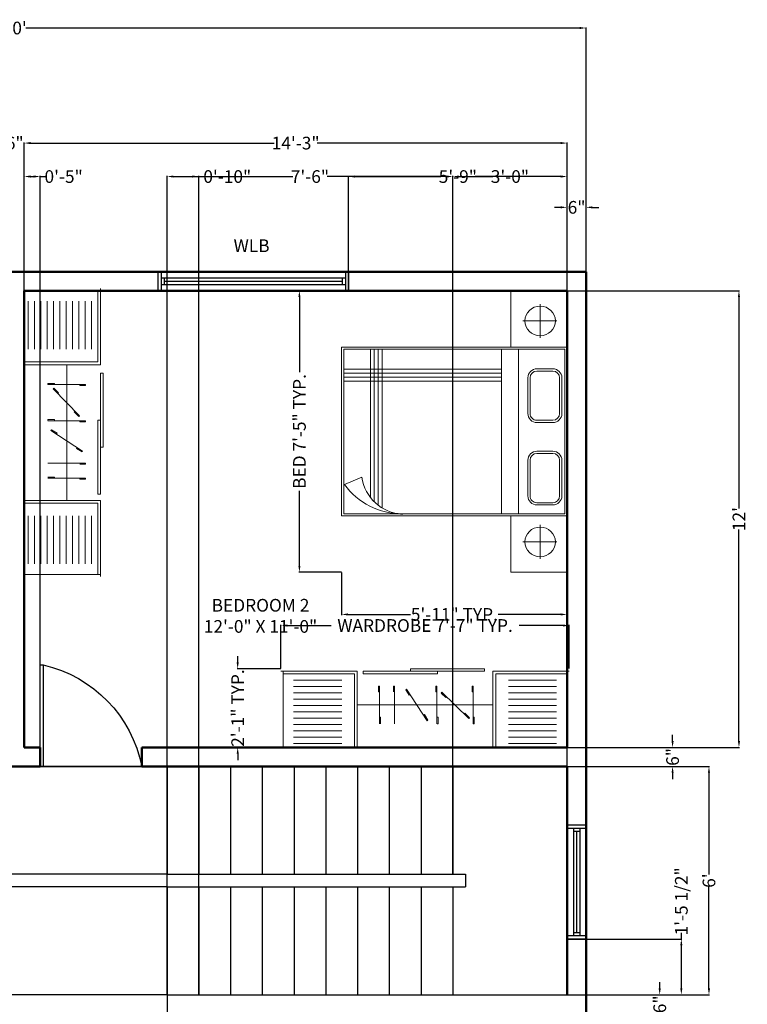
# Model space of a CAD drawing. Units: inches. Extents: x 2663 to 3147, y 140 to 736.
# Tile 6 of 6: x 2918 to 3147, y 425 to 736. Entities that reach past the tile are written whole.
import ezdxf

# ---------------------------------------------------------------- set-up
doc = ezdxf.new("R2010")
doc.units = ezdxf.units.IN
doc.header["$MEASUREMENT"] = 0
for name, color, linetype, lineweight in [('A-ANNO-DIMS', 2, 'Continuous', 18), ('A-AREA-IDEN', 3, 'Continuous', 25), ('A-DOOR', 3, 'Continuous', 25), ('A-FLOR-STRS', 1, 'Continuous', 25), ('A-FURN', 8, 'Continuous', 18), ('A-GLAZ', 4, 'Continuous', 25), ('A-WALL', 7, 'Continuous', 50)]:
    doc.layers.add(name, color=color, linetype=linetype, lineweight=lineweight)
doc.styles.get("Standard").update_dxf_attribs({"font": 'arial.ttf'})
doc.dimstyles.get("Standard").update_dxf_attribs({"dimtxt": 4, "dimasz": 2, "dimexe": 0.18, "dimexo": 0.0625, "dimgap": 0.09, "dimtad": 0, "dimdec": 0, "dimzin": 0, "dimdsep": 46, "dimlunit": 4, "dimtxsty": 'Standard', "dimcen": 0.09, "dimadec": 0, "dimazin": 0, "dimtfac": 1, "dimtdec": 0, "dimtofl": 0, "dimtmove": 0, "dimatfit": 3, "dimfxl": 1, "dimtolj": 1, "dimtzin": 0, "dimarcsym": 0})

# ---------------------------------------------------------------- blocks, each defined once
blk = doc.blocks.new('*D2')
at = {"layer": 'A-ANNO-DIMS', "color": 0, "lineweight": -2, "transparency": 16777216}
for p, q in [((2911.16, 696.87), (2909.16, 696.87)), ((2913.16, 650.39), (2913.16, 697.05)), ((2919.16, 650.39), (2919.16, 697.05)), ((2921.16, 696.87), (2923.16, 696.87))]:
    blk.add_line(p, q, dxfattribs=at)
at = {"layer": 'A-ANNO-DIMS', "color": 0, "transparency": 16777216}
for points in [[(2911.16, 697.21), (2911.16, 696.54), (2913.16, 696.87)], [(2921.16, 697.21), (2921.16, 696.54), (2919.16, 696.87)]]:
    blk.add_solid(points, dxfattribs=at)
at = {"layer": 'Defpoints', "color": 0, "transparency": 16777216}
for p in [(2919.16, 696.87), (2913.16, 650.32), (2919.16, 650.32)]:
    blk.add_point(p, dxfattribs=at)
at = {"layer": 'A-ANNO-DIMS', "color": 0, "transparency": 16777216, "insert": (2916.16, 696.87), "char_height": 4, "attachment_point": 5}
blk.add_mtext('\\A1;6"', dxfattribs=at)
blk = doc.blocks.new('*D3')
at = {"layer": 'A-ANNO-DIMS', "color": 0, "lineweight": -2, "transparency": 16777216}
for p, q in [((2919.16, 650.39), (2919.16, 697.05)), ((2921.16, 696.87), (2997.89, 696.87)), ((3088.16, 696.87), (3011.43, 696.87)), ((3090.16, 650.39), (3090.16, 697.05))]:
    blk.add_line(p, q, dxfattribs=at)
at = {"layer": 'A-ANNO-DIMS', "color": 0, "transparency": 16777216}
for points in [[(2921.16, 697.21), (2921.16, 696.54), (2919.16, 696.87)], [(3088.16, 697.21), (3088.16, 696.54), (3090.16, 696.87)]]:
    blk.add_solid(points, dxfattribs=at)
at = {"layer": 'Defpoints', "color": 0, "transparency": 16777216}
for p in [(3090.16, 696.87), (2919.16, 650.32), (3090.16, 650.32)]:
    blk.add_point(p, dxfattribs=at)
at = {"layer": 'A-ANNO-DIMS', "color": 0, "transparency": 16777216, "insert": (3004.66, 696.87), "char_height": 4, "attachment_point": 5}
blk.add_mtext('\\A1;14\'-3"', dxfattribs=at)
blk = doc.blocks.new('*D7')
at = {"layer": 'A-ANNO-DIMS', "color": 0, "lineweight": -2, "transparency": 16777216}
for p, q in [((3090.22, 500.32), (3135.04, 500.32)), ((3134.86, 498.32), (3134.86, 466.26)), ((3134.86, 430.32), (3134.86, 462.38)), ((3090.22, 428.32), (3135.04, 428.32))]:
    blk.add_line(p, q, dxfattribs=at)
at = {"layer": 'A-ANNO-DIMS', "color": 0, "transparency": 16777216}
for points in [[(3134.53, 498.32), (3135.2, 498.32), (3134.86, 500.32)], [(3134.53, 430.32), (3135.2, 430.32), (3134.86, 428.32)]]:
    blk.add_solid(points, dxfattribs=at)
at = {"layer": 'Defpoints', "color": 0, "transparency": 16777216}
for p in [(3090.16, 500.32), (3090.16, 428.32), (3134.86, 428.32)]:
    blk.add_point(p, dxfattribs=at)
at = {"layer": 'A-ANNO-DIMS', "color": 0, "transparency": 16777216, "insert": (3134.86, 464.32), "char_height": 4, "attachment_point": 5, "rotation": 90}
blk.add_mtext("\\A1;6'", dxfattribs=at)
blk = doc.blocks.new('EDFRTYUI')
for p, q in [((3325.9, 253.54), (3325.9, 259.54)), ((3325.9, 259.54), (3385.9, 259.54)), ((3326.9, 253.54), (3326.9, 259.54)), ((3384.9, 259.54), (3384.9, 253.54)), ((3385.9, 259.54), (3385.9, 253.54)), ((3326.9, 257.54), (3384.9, 257.54)), ((3326.9, 255.54), (3384.9, 255.54)), ((3327.9, 255.54), (3327.9, 257.54)), ((3327.9, 256.54), (3383.9, 256.54)), ((3383.9, 257.54), (3383.9, 255.54)), ((3385.9, 253.54), (3325.9, 253.54))]:
    blk.add_line(p, q)
at = {"insert": (3337.87, 269.72), "char_height": 4, "attachment_point": 1}
blk.add_mtext_dynamic_manual_height_columns('\\pxqc;WLB', width=34.9199, gutter_width=20, heights=[0], dxfattribs=at)
blk = doc.blocks.new('FGCHBJK')
for p, q in [((3315.88, 342.07), (3315.88, 348.07)), ((3315.88, 348.07), (3351.88, 348.07)), ((3316.88, 342.07), (3316.88, 348.07)), ((3350.88, 348.07), (3350.88, 342.07)), ((3351.88, 348.07), (3351.88, 342.07)), ((3316.88, 346.07), (3350.88, 346.07)), ((3317.88, 344.07), (3317.88, 346.07)), ((3317.88, 345.07), (3349.88, 345.07)), ((3349.88, 346.07), (3349.88, 344.07)), ((3351.88, 342.07), (3315.88, 342.07)), ((3316.88, 344.07), (3350.88, 344.07))]:
    blk.add_line(p, q)
blk = doc.blocks.new('A$C057D194F')
for p, q in [((0, 1.5, -0.1688), (0, 2, -0.1688)), ((0, 2, -0.1688), (0.5, 2, -0.1688)), ((0.5, 2, -0.1688), (0.5, 0, -0.1688)), ((2, 2, -0.1688), (0.5, 2, -0.1688)), ((1.98, 1.98, -0.1688), (0.52, 1.98, -0.1688)), ((0.52, 1.98, -0.1688), (0.52, 0.02, -0.1688)), ((1.0907, 1.9539, -0.1688), (0.7735, 1.9539, -0.1688)), ((1.0907, 1.9339, -0.1688), (0.7735, 1.9339, -0.1688)), ((1.8224, 1.9539, -0.1688), (1.5052, 1.9539, -0.1688)), ((1.8224, 1.9339, -0.1688), (1.5052, 1.9339, -0.1688)), ((1.98, 0.02, -0.1688), (1.98, 1.98, -0.1688)), ((2, 0, -0.1688), (2, 2, -0.1688)), ((2.5, 2, -0.1688), (2, 2, -0.1688)), ((2.5, 1.5, -0.1688), (2.5, 2, -0.1688)), ((0.2687, 1.9081, -0.1688), (0.2687, 1.761, -0.1688)), ((0.2687, 1.6081, -0.1688), (0.2687, 1.9081, -0.1688)), ((0.6935, 1.8739, -0.1688), (0.6935, 1.7322, -0.1688)), ((0.7135, 1.8739, -0.1688), (0.7135, 1.7322, -0.1688)), ((1.1507, 1.7322, -0.1688), (1.1507, 1.8739, -0.1688)), ((1.1707, 1.7322, -0.1688), (1.1707, 1.8739, -0.1688)), ((1.4252, 1.8739, -0.1688), (1.4252, 1.7322, -0.1688)), ((1.4452, 1.8739, -0.1688), (1.4452, 1.7322, -0.1688)), ((1.8824, 1.7322, -0.1688), (1.8824, 1.8739, -0.1688)), ((1.9024, 1.7322, -0.1688), (1.9024, 1.8739, -0.1688)), ((2.2313, 1.9081, -0.1688), (2.2313, 1.761, -0.1688)), ((2.2313, 1.6081, -0.1688), (2.2313, 1.9081, -0.1688)), ((0.4194, 1.761, -0.1688), (0.1194, 1.761, -0.1688)), ((0.2687, 1.761, -0.1688), (0.4194, 1.761, -0.1688)), ((0.2687, 1.761, -0.1688), (0.2687, 1.6081, -0.1688)), ((2.0806, 1.761, -0.1688), (2.3806, 1.761, -0.1688)), ((2.2313, 1.761, -0.1688), (2.0806, 1.761, -0.1688)), ((2.2313, 1.761, -0.1688), (2.2313, 1.6081, -0.1688)), ((0.7735, 1.6722, -0.1688), (1.0907, 1.6722, -0.1688)), ((1.5052, 1.6722, -0.1688), (1.8224, 1.6722, -0.1688)), ((0.7735, 1.6522, -0.1688), (1.0907, 1.6522, -0.1688)), ((1.5052, 1.6522, -0.1688), (1.8224, 1.6522, -0.1688)), ((0.5, 1.5, -0.1688), (0, 1.5, -0.1688)), ((1.98, 1.5693, -0.1688), (0.52, 1.5693, -0.1688)), ((2, 1.5, -0.1688), (2.5, 1.5, -0.1688)), ((1.98, 1.4193, -0.1688), (0.52, 1.4193, -0.1688)), ((0.6969, 0.02, -0.1688), (0.6969, 1.4193, -0.1688)), ((0.7319, 0.02, -0.1688), (0.7319, 1.4193, -0.1688)), ((0.7669, 0.02, -0.1688), (0.7669, 1.4193, -0.1688)), ((0.8019, 0.02, -0.1688), (0.8019, 1.4193, -0.1688)), ((0.52, 0.3595, -0.1688), (1.9292, 0.3595, -0.1688)), ((0.52, 0.3245, -0.1688), (1.905, 0.3245, -0.1688)), ((0.52, 0.2895, -0.1688), (1.8742, 0.2895, -0.1688)), ((0.52, 0.2545, -0.1688), (1.8344, 0.2545, -0.1688)), ((1.6548, 0.1789, -0.1688), (1.7198, 0.0251, -0.1688)), ((0.52, 0.02, -0.1688), (1.98, 0.02, -0.1688)), ((0.5, 0, -0.1688), (2, 0, -0.1688))]:
    blk.add_line(p, q)
for centre, radius, start, end in [((0.7735, 1.8739, -0.1688), 0.08, 90, 180), ((0.7735, 1.8739, -0.1688), 0.06, 90, 180), ((1.0907, 1.8739, -0.1688), 0.08, 0, 90), ((1.0907, 1.8739, -0.1688), 0.06, 0, 90), ((1.5052, 1.8739, -0.1688), 0.08, 90, 180), ((1.5052, 1.8739, -0.1688), 0.06, 90, 180), ((1.8224, 1.8739, -0.1688), 0.08, 0, 90), ((1.8224, 1.8739, -0.1688), 0.06, 0, 90), ((0.7735, 1.7322, -0.1688), 0.08, 180, 270), ((0.7735, 1.7322, -0.1688), 0.06, 180, 270), ((1.0907, 1.7322, -0.1688), 0.08, 270, 0), ((1.0907, 1.7322, -0.1688), 0.06, 270, 0), ((1.5052, 1.7322, -0.1688), 0.08, 180, 270), ((1.5052, 1.7322, -0.1688), 0.06, 180, 270), ((1.8224, 1.7322, -0.1688), 0.08, 270, 0), ((1.8224, 1.7322, -0.1688), 0.06, 270, 0), ((1.5992, 0.5623, -0.1688), 0.3874, 278.2518, 356.6808), ((1.363, 0.5286, -0.1688), 0.6171, 305.32946, 1.04595)]:
    blk.add_arc(centre, radius, start, end)
blk.add_ellipse((0.2687, 1.761, -0.1688), major_axis=(0, -0.1351), ratio=0.975448)
at = {"extrusion": (0, 0, -1)}
blk.add_ellipse((2.2313, 1.761, -0.1688), major_axis=(0, 0.1351), ratio=0.975448, dxfattribs=at)
for p in [(0.2687, 1.761, -0.1688), (2.2313, 1.761, -0.1688)]:
    blk.add_point(p)
blk = doc.blocks.new('A$C34930FF8')
at = {"ltscale": 0.05}
for p, q in [((0, 2252.4), (0, 16.8)), ((600, 2252.4), (0, 2252.4)), ((185.4, 1513), (185.4, 1521.5)), ((227.1, 1479.2), (233.2, 1485.2)), ((237.7, 1513), (237.7, 1521.5)), ((436.7, 1513), (436.7, 1504.4)), ((482.5, 1513), (482.5, 1504.4)), ((263.6, 1441.7), (269.7, 1447.7)), ((398.2, 1303.6), (392.1, 1297.6)), ((434.8, 1266.1), (428.7, 1260.1)), ((185.4, 1229.1), (185.4, 1237.7)), ((237.7, 1229.1), (237.7, 1237.7)), ((436.7, 1228.2), (436.7, 1219.7)), ((482.5, 1228.2), (482.5, 1219.7)), ((209.5, 1150.1), (214.1, 1157.3)), ((253.5, 1121.8), (258.1, 1129)), ((415.3, 1017.6), (410.6, 1010.5)), ((459.3, 989.3), (454.7, 982.1)), ((482.5, 894.9), (482.5, 886.3)), ((237.7, 775.3), (237.7, 783.9)), ((436.7, 775.3), (436.7, 766.8)), ((482.5, 775.3), (482.5, 766.8)), ((600, 16.8), (0, 16.8))]:
    blk.add_line(p, q, dxfattribs=at)
for p, q in [((580, 1690.9), (580, 2252.4)), ((600, 1669.3), (600, 2269.3)), ((30, 1790.9), (30, 2169.3)), ((80, 1790.9), (80, 2169.3)), ((130, 1790.9), (130, 2169.3)), ((180, 1790.9), (180, 2169.3)), ((230, 1790.9), (230, 2169.3)), ((280, 1790.9), (280, 2169.3)), ((330, 1790.9), (330, 2169.3)), ((380, 1790.9), (380, 2169.3)), ((430, 1790.9), (430, 2169.3)), ((480, 1790.9), (480, 2169.3)), ((530, 1790.9), (530, 2169.3)), ((580, 1690.9), (0, 1690.9)), ((600, 1669.3), (0, 1669.3)), ((335.4, 1666.1), (335.4, 603.1)), ((600, 1603.3), (620, 1603.3)), ((600, 1018.7), (600, 1603.3)), ((620, 1603.3), (620, 1018.7)), ((237.7, 1521.5), (185.4, 1521.5)), ((482.5, 1513), (185.4, 1513)), ((434.8, 1266.1), (227.4, 1478.9)), ((269.7, 1447.7), (233.2, 1485.2)), ((436.7, 1504.4), (482.5, 1504.4)), ((428.7, 1260.1), (392.1, 1297.6)), ((237.7, 1237.7), (185.4, 1237.7)), ((482.5, 1228.2), (185.4, 1228.2)), ((436.7, 1219.7), (482.5, 1219.7)), ((600, 1233.4), (580, 1233.4)), ((580, 1233.4), (580, 648.7)), ((600, 648.7), (600, 1233.4)), ((459.3, 989.3), (209.5, 1150.1)), ((258.1, 1129), (214.1, 1157.3)), ((454.7, 982.1), (410.6, 1010.5)), ((620, 1018.7), (600, 1018.7)), ((482.5, 894.9), (185.4, 894.9)), ((436.7, 886.3), (482.5, 886.3)), ((237.7, 783.9), (185.4, 783.9)), ((482.5, 775.3), (185.4, 775.3)), ((436.7, 766.8), (482.5, 766.8)), ((580, 648.7), (600, 648.7)), ((600, 600), (0, 600)), ((580, 578.3), (0, 578.3)), ((580, 578.3), (580, 16.8)), ((600, 600), (600, 0)), ((30, 478.3), (30, 100)), ((80, 478.3), (80, 100)), ((130, 478.3), (130, 100)), ((180, 478.3), (180, 100)), ((230, 478.3), (230, 100)), ((280, 478.3), (280, 100)), ((330, 478.3), (330, 100)), ((380, 478.3), (380, 100)), ((430, 478.3), (430, 100)), ((480, 478.3), (480, 100)), ((530, 478.3), (530, 100))]:
    blk.add_line(p, q)
blk = doc.blocks.new('DXFGVHBJKL')
for p, q in [((2908.16, 532.32), (2907.16, 532.32)), ((2907.16, 532.32), (2907.16, 500.32)), ((2908.16, 500.32), (2908.16, 532.32)), ((2908.16, 500.32), (2876.16, 500.32))]:
    blk.add_line(p, q)
blk.add_arc((2916.21, 492.54), 40.8, 102.812, 169.0067)
blk = doc.blocks.new('*D22')
at = {"layer": 'A-ANNO-DIMS', "color": 0, "lineweight": -2, "transparency": 16777216}
for p, q in [((3090.16, 656.39), (3090.16, 676.79)), ((3096.16, 656.39), (3096.16, 676.79)), ((3088.16, 676.61), (3086.16, 676.61)), ((3098.16, 676.61), (3100.16, 676.61))]:
    blk.add_line(p, q, dxfattribs=at)
at = {"layer": 'A-ANNO-DIMS', "color": 0, "transparency": 16777216}
for points in [[(3088.16, 676.94), (3088.16, 676.28), (3090.16, 676.61)], [(3098.16, 676.94), (3098.16, 676.28), (3096.16, 676.61)]]:
    blk.add_solid(points, dxfattribs=at)
at = {"layer": 'Defpoints', "color": 0, "transparency": 16777216}
for p in [(3090.16, 676.61), (3090.16, 656.32), (3096.16, 656.32)]:
    blk.add_point(p, dxfattribs=at)
at = {"layer": 'A-ANNO-DIMS', "color": 0, "transparency": 16777216, "insert": (3093.16, 676.61), "char_height": 4, "attachment_point": 5}
blk.add_mtext('\\A1;6"', dxfattribs=at)
blk = doc.blocks.new('*D23')
at = {"layer": 'A-ANNO-DIMS', "color": 0, "lineweight": -2, "transparency": 16777216}
for p, q in [((3090.22, 650.32), (3144.49, 650.32)), ((3144.31, 648.32), (3144.31, 581.62)), ((3144.31, 508.32), (3144.31, 575.03)), ((3090.22, 506.32), (3144.49, 506.32))]:
    blk.add_line(p, q, dxfattribs=at)
at = {"layer": 'A-ANNO-DIMS', "color": 0, "transparency": 16777216}
for points in [[(3143.98, 648.32), (3144.65, 648.32), (3144.31, 650.32)], [(3143.98, 508.32), (3144.65, 508.32), (3144.31, 506.32)]]:
    blk.add_solid(points, dxfattribs=at)
at = {"layer": 'Defpoints', "color": 0, "transparency": 16777216}
for p in [(3090.16, 650.32), (3090.16, 506.32), (3144.31, 506.32)]:
    blk.add_point(p, dxfattribs=at)
at = {"layer": 'A-ANNO-DIMS', "color": 0, "transparency": 16777216, "insert": (3144.31, 578.32), "char_height": 4, "attachment_point": 5, "rotation": 90}
blk.add_mtext("\\A1;12'", dxfattribs=at)
blk = doc.blocks.new('*D24')
at = {"layer": 'A-ANNO-DIMS', "color": 0, "lineweight": -2, "transparency": 16777216}
for p, q in [((3123.4, 508.32), (3123.4, 510.32)), ((3096.22, 506.32), (3123.58, 506.32)), ((3096.22, 500.32), (3123.58, 500.32)), ((3123.4, 498.32), (3123.4, 496.32))]:
    blk.add_line(p, q, dxfattribs=at)
at = {"layer": 'A-ANNO-DIMS', "color": 0, "transparency": 16777216}
for points in [[(3123.07, 508.32), (3123.74, 508.32), (3123.4, 506.32)], [(3123.07, 498.32), (3123.74, 498.32), (3123.4, 500.32)]]:
    blk.add_solid(points, dxfattribs=at)
at = {"layer": 'Defpoints', "color": 0, "transparency": 16777216}
for p in [(3096.16, 506.32), (3096.16, 500.32), (3123.4, 500.32)]:
    blk.add_point(p, dxfattribs=at)
at = {"layer": 'A-ANNO-DIMS', "color": 0, "transparency": 16777216, "insert": (3123.4, 503.32), "char_height": 4, "attachment_point": 5, "rotation": 90}
blk.add_mtext('\\A1;6"', dxfattribs=at)
blk = doc.blocks.new('*D25')
at = {"layer": 'A-ANNO-DIMS', "color": 0, "lineweight": -2, "transparency": 16777216}
for p, q in [((3119.35, 430.32), (3119.35, 432.32)), ((3096.22, 428.32), (3119.53, 428.32)), ((3096.22, 422.32), (3119.53, 422.32)), ((3119.35, 420.32), (3119.35, 418.32))]:
    blk.add_line(p, q, dxfattribs=at)
at = {"layer": 'A-ANNO-DIMS', "color": 0, "transparency": 16777216}
for points in [[(3119.01, 430.32), (3119.68, 430.32), (3119.35, 428.32)], [(3119.01, 420.32), (3119.68, 420.32), (3119.35, 422.32)]]:
    blk.add_solid(points, dxfattribs=at)
at = {"layer": 'Defpoints', "color": 0, "transparency": 16777216}
for p in [(3096.16, 428.32), (3096.16, 422.32), (3119.35, 422.32)]:
    blk.add_point(p, dxfattribs=at)
at = {"layer": 'A-ANNO-DIMS', "color": 0, "transparency": 16777216, "insert": (3119.35, 425.32), "char_height": 4, "attachment_point": 5, "rotation": 90}
blk.add_mtext('\\A1;6"', dxfattribs=at)
blk = doc.blocks.new('*D38')
at = {"layer": 'A-ANNO-DIMS', "color": 0, "lineweight": -2, "transparency": 16777216}
for p, q in [((2736.16, 656.39), (2736.16, 733.33)), ((2738.16, 733.15), (2912.68, 733.15)), ((3094.16, 733.15), (2919.64, 733.15)), ((3096.16, 656.39), (3096.16, 733.33))]:
    blk.add_line(p, q, dxfattribs=at)
at = {"layer": 'A-ANNO-DIMS', "color": 0, "transparency": 16777216}
for points in [[(2738.16, 733.48), (2738.16, 732.82), (2736.16, 733.15)], [(3094.16, 733.48), (3094.16, 732.82), (3096.16, 733.15)]]:
    blk.add_solid(points, dxfattribs=at)
at = {"layer": 'Defpoints', "color": 0, "transparency": 16777216}
for p in [(3096.16, 733.15), (2736.16, 656.32), (3096.16, 656.32)]:
    blk.add_point(p, dxfattribs=at)
at = {"layer": 'A-ANNO-DIMS', "color": 0, "transparency": 16777216, "insert": (2916.16, 733.15), "char_height": 4, "attachment_point": 5}
blk.add_mtext("\\A1;30'", dxfattribs=at)
blk = doc.blocks.new('*D39')
at = {"layer": 'A-ANNO-DIMS', "color": 0, "lineweight": -2, "transparency": 16777216}
for p, q in [((2912.96, 532.32), (2912.96, 534.32)), ((2908.22, 532.32), (2913.14, 532.32)), ((2912.96, 502.32), (2912.96, 530.32)), ((2908.22, 500.32), (2913.14, 500.32))]:
    blk.add_line(p, q, dxfattribs=at)
at = {"layer": 'A-ANNO-DIMS', "color": 0, "transparency": 16777216}
for points in [[(2912.63, 530.32), (2913.29, 530.32), (2912.96, 532.32)], [(2912.63, 502.32), (2913.29, 502.32), (2912.96, 500.32)]]:
    blk.add_solid(points, dxfattribs=at)
at = {"layer": 'Defpoints', "color": 0, "transparency": 16777216}
for p in [(2908.16, 532.32), (2912.96, 532.32), (2908.16, 500.32)]:
    blk.add_point(p, dxfattribs=at)
at = {"layer": 'A-ANNO-DIMS', "color": 0, "transparency": 16777216, "insert": (2912.96, 555.66), "char_height": 4, "attachment_point": 5, "rotation": 90}
blk.add_mtext('\\A1;DOOR 2\'-8" TYP.', dxfattribs=at)
blk = doc.blocks.new('*D45')
at = {"layer": 'A-ANNO-DIMS', "color": 0, "lineweight": -2, "transparency": 16777216}
for p, q in [((3000.02, 531.2), (3000.02, 544.94)), ((3002.02, 544.76), (3015.84, 544.76)), ((3088.84, 544.76), (3075.02, 544.76)), ((3090.84, 531.2), (3090.84, 544.94))]:
    blk.add_line(p, q, dxfattribs=at)
at = {"layer": 'A-ANNO-DIMS', "color": 0, "transparency": 16777216}
for points in [[(3002.02, 545.09), (3002.02, 544.42), (3000.02, 544.76)], [(3088.84, 545.09), (3088.84, 544.42), (3090.84, 544.76)]]:
    blk.add_solid(points, dxfattribs=at)
at = {"layer": 'Defpoints', "color": 0, "transparency": 16777216}
for p in [(3090.84, 544.76), (3000.02, 531.14), (3090.84, 531.14)]:
    blk.add_point(p, dxfattribs=at)
at = {"layer": 'A-ANNO-DIMS', "color": 0, "transparency": 16777216, "insert": (3045.43, 544.76), "char_height": 4, "attachment_point": 5}
blk.add_mtext('\\A1;WARDROBE 7\'-7" TYP.', dxfattribs=at)
blk = doc.blocks.new('*D46')
at = {"layer": 'A-ANNO-DIMS', "color": 0, "lineweight": -2, "transparency": 16777216}
for p, q in [((2986.4, 533.14), (2986.4, 535.14)), ((2999.96, 531.14), (2986.22, 531.14)), ((2999.96, 506.32), (2986.22, 506.32)), ((2986.4, 504.32), (2986.4, 502.32))]:
    blk.add_line(p, q, dxfattribs=at)
at = {"layer": 'A-ANNO-DIMS', "color": 0, "transparency": 16777216}
for points in [[(2986.07, 533.14), (2986.73, 533.14), (2986.4, 531.14)], [(2986.07, 504.32), (2986.73, 504.32), (2986.4, 506.32)]]:
    blk.add_solid(points, dxfattribs=at)
at = {"layer": 'Defpoints', "color": 0, "transparency": 16777216}
for p in [(2986.4, 531.14), (3000.02, 531.14), (3000.02, 506.32)]:
    blk.add_point(p, dxfattribs=at)
at = {"layer": 'A-ANNO-DIMS', "color": 0, "transparency": 16777216, "insert": (2986.4, 518.73), "char_height": 4, "attachment_point": 5, "rotation": 90}
blk.add_mtext('\\A1;2\'-1" TYP.', dxfattribs=at)
blk = doc.blocks.new('*D47')
at = {"layer": 'A-ANNO-DIMS', "color": 0, "lineweight": -2, "transparency": 16777216}
for p, q in [((3019.09, 650.32), (3005.66, 650.32)), ((3005.84, 648.32), (3005.84, 624.66)), ((3005.84, 563.56), (3005.84, 587.23)), ((3019.09, 561.56), (3005.66, 561.56))]:
    blk.add_line(p, q, dxfattribs=at)
at = {"layer": 'A-ANNO-DIMS', "color": 0, "transparency": 16777216}
for points in [[(3005.51, 648.32), (3006.17, 648.32), (3005.84, 650.32)], [(3005.51, 563.56), (3006.17, 563.56), (3005.84, 561.56)]]:
    blk.add_solid(points, dxfattribs=at)
at = {"layer": 'Defpoints', "color": 0, "transparency": 16777216}
for p in [(3019.15, 650.32), (3005.84, 561.56), (3019.15, 561.56)]:
    blk.add_point(p, dxfattribs=at)
at = {"layer": 'A-ANNO-DIMS', "color": 0, "transparency": 16777216, "insert": (3005.84, 605.94), "char_height": 4, "attachment_point": 5, "rotation": 90}
blk.add_mtext('\\A1;BED 7\'-5" TYP.', dxfattribs=at)
blk = doc.blocks.new('*D48')
at = {"layer": 'A-ANNO-DIMS', "color": 0, "lineweight": -2, "transparency": 16777216}
for p, q in [((3019.15, 561.5), (3019.15, 548.07)), ((3090.16, 561.5), (3090.16, 548.07)), ((3021.15, 548.25), (3040.82, 548.25)), ((3088.16, 548.25), (3068.49, 548.25))]:
    blk.add_line(p, q, dxfattribs=at)
at = {"layer": 'A-ANNO-DIMS', "color": 0, "transparency": 16777216}
for points in [[(3021.15, 548.58), (3021.15, 547.92), (3019.15, 548.25)], [(3088.16, 548.58), (3088.16, 547.92), (3090.16, 548.25)]]:
    blk.add_solid(points, dxfattribs=at)
at = {"layer": 'Defpoints', "color": 0, "transparency": 16777216}
for p in [(3019.15, 561.56), (3090.16, 561.56), (3090.16, 548.25)]:
    blk.add_point(p, dxfattribs=at)
at = {"layer": 'A-ANNO-DIMS', "color": 0, "transparency": 16777216, "insert": (3054.66, 548.25), "char_height": 4, "attachment_point": 5}
blk.add_mtext('\\A1;5\'-11" TYP.', dxfattribs=at)
blk = doc.blocks.new('*D66')
at = {"layer": 'A-ANNO-DIMS', "color": 0, "lineweight": -2, "transparency": 16777216}
for p, q in [((2964.16, 466.39), (2964.16, 686.5)), ((2966.16, 686.32), (3003.77, 686.32)), ((3052.16, 686.32), (3014.55, 686.32)), ((3054.16, 466.39), (3054.16, 686.5))]:
    blk.add_line(p, q, dxfattribs=at)
at = {"layer": 'A-ANNO-DIMS', "color": 0, "transparency": 16777216}
for points in [[(2966.16, 686.66), (2966.16, 685.99), (2964.16, 686.32)], [(3052.16, 686.66), (3052.16, 685.99), (3054.16, 686.32)]]:
    blk.add_solid(points, dxfattribs=at)
at = {"layer": 'Defpoints', "color": 0, "transparency": 16777216}
for p in [(3054.16, 686.32), (2964.16, 466.32), (3054.16, 466.32)]:
    blk.add_point(p, dxfattribs=at)
at = {"layer": 'A-ANNO-DIMS', "color": 0, "transparency": 16777216, "insert": (3009.16, 686.32), "char_height": 4, "attachment_point": 5}
blk.add_mtext('\\A1;7\'-6"', dxfattribs=at)
blk = doc.blocks.new('*D67')
at = {"layer": 'A-ANNO-DIMS', "color": 0, "lineweight": -2, "transparency": 16777216}
for p, q in [((3054.16, 466.39), (3054.16, 686.5)), ((3056.16, 686.32), (3066.76, 686.32)), ((3088.16, 686.32), (3077.57, 686.32)), ((3090.16, 428.39), (3090.16, 686.5))]:
    blk.add_line(p, q, dxfattribs=at)
at = {"layer": 'A-ANNO-DIMS', "color": 0, "transparency": 16777216}
for points in [[(3056.16, 686.66), (3056.16, 685.99), (3054.16, 686.32)], [(3088.16, 686.66), (3088.16, 685.99), (3090.16, 686.32)]]:
    blk.add_solid(points, dxfattribs=at)
at = {"layer": 'Defpoints', "color": 0, "transparency": 16777216}
for p in [(3090.16, 686.32), (3054.16, 466.32), (3090.16, 428.32)]:
    blk.add_point(p, dxfattribs=at)
at = {"layer": 'A-ANNO-DIMS', "color": 0, "transparency": 16777216, "insert": (3072.16, 686.32), "char_height": 4, "attachment_point": 5}
blk.add_mtext('\\A1;3\'-0"', dxfattribs=at)
blk = doc.blocks.new('*D69')
at = {"layer": 'A-ANNO-DIMS', "color": 0, "lineweight": -2, "transparency": 16777216}
for p, q in [((3021.35, 650.39), (3021.35, 686.5)), ((3023.35, 686.32), (3050.35, 686.32)), ((3088.16, 686.32), (3061.16, 686.32)), ((3090.16, 650.39), (3090.16, 686.5))]:
    blk.add_line(p, q, dxfattribs=at)
at = {"layer": 'A-ANNO-DIMS', "color": 0, "transparency": 16777216}
for points in [[(3023.35, 686.66), (3023.35, 685.99), (3021.35, 686.32)], [(3088.16, 686.66), (3088.16, 685.99), (3090.16, 686.32)]]:
    blk.add_solid(points, dxfattribs=at)
at = {"layer": 'Defpoints', "color": 0, "transparency": 16777216}
for p in [(3090.16, 686.32), (3021.35, 650.32), (3090.16, 650.32)]:
    blk.add_point(p, dxfattribs=at)
at = {"layer": 'A-ANNO-DIMS', "color": 0, "transparency": 16777216, "insert": (3055.76, 686.32), "char_height": 4, "attachment_point": 5}
blk.add_mtext('\\A1;5\'-9"', dxfattribs=at)
blk = doc.blocks.new('*D74')
at = {"layer": 'A-ANNO-DIMS', "color": 0, "lineweight": -2, "transparency": 16777216}
for p, q in [((3126.16, 445.91), (3126.16, 447.91)), ((3090.22, 445.91), (3126.34, 445.91)), ((3126.16, 430.32), (3126.16, 443.91)), ((3090.22, 428.32), (3126.34, 428.32))]:
    blk.add_line(p, q, dxfattribs=at)
at = {"layer": 'A-ANNO-DIMS', "color": 0, "transparency": 16777216}
for points in [[(3125.83, 443.91), (3126.49, 443.91), (3126.16, 445.91)], [(3125.83, 430.32), (3126.49, 430.32), (3126.16, 428.32)]]:
    blk.add_solid(points, dxfattribs=at)
at = {"layer": 'Defpoints', "color": 0, "transparency": 16777216}
for p in [(3090.16, 445.91), (3126.16, 445.91), (3090.16, 428.32)]:
    blk.add_point(p, dxfattribs=at)
at = {"layer": 'A-ANNO-DIMS', "color": 0, "transparency": 16777216, "insert": (3126.16, 457.79), "char_height": 4, "attachment_point": 5, "rotation": 90}
blk.add_mtext('\\A1;1\'-5 1/2"', dxfattribs=at)
blk = doc.blocks.new('*D76')
at = {"layer": 'A-ANNO-DIMS', "color": 0, "lineweight": -2, "transparency": 16777216}
for p, q in [((2919.16, 506.39), (2919.16, 686.5)), ((2921.16, 686.32), (2922.16, 686.32)), ((2924.16, 506.39), (2924.16, 686.5)), ((2924.16, 686.32), (2926.16, 686.32))]:
    blk.add_line(p, q, dxfattribs=at)
at = {"layer": 'A-ANNO-DIMS', "color": 0, "transparency": 16777216}
for points in [[(2921.16, 686.66), (2921.16, 685.99), (2919.16, 686.32)], [(2922.16, 686.66), (2922.16, 685.99), (2924.16, 686.32)]]:
    blk.add_solid(points, dxfattribs=at)
at = {"layer": 'Defpoints', "color": 0, "transparency": 16777216}
for p in [(2924.16, 686.32), (2919.16, 506.32), (2924.16, 506.32)]:
    blk.add_point(p, dxfattribs=at)
at = {"layer": 'A-ANNO-DIMS', "color": 0, "transparency": 16777216, "insert": (2931.57, 686.32), "char_height": 4, "attachment_point": 5}
blk.add_mtext('\\A1;0\'-5"', dxfattribs=at)
blk = doc.blocks.new('*D85')
at = {"layer": 'A-ANNO-DIMS', "color": 0, "lineweight": -2, "transparency": 16777216}
for p, q in [((2964.1, 462.32), (2705.98, 462.32)), ((2706.16, 460.32), (2706.16, 452.32)), ((2706.16, 430.32), (2706.16, 438.33)), ((2964.1, 428.32), (2705.98, 428.32))]:
    blk.add_line(p, q, dxfattribs=at)
at = {"layer": 'A-ANNO-DIMS', "color": 0, "transparency": 16777216}
for points in [[(2705.83, 460.32), (2706.49, 460.32), (2706.16, 462.32)], [(2705.83, 430.32), (2706.49, 430.32), (2706.16, 428.32)]]:
    blk.add_solid(points, dxfattribs=at)
at = {"layer": 'Defpoints', "color": 0, "transparency": 16777216}
for p in [(2706.16, 462.32), (2964.16, 462.32), (2964.16, 428.32)]:
    blk.add_point(p, dxfattribs=at)
at = {"layer": 'A-ANNO-DIMS', "color": 0, "transparency": 16777216, "insert": (2706.16, 445.32), "char_height": 4, "attachment_point": 5, "rotation": 90}
blk.add_mtext('\\A1;2\'-10"', dxfattribs=at)
blk = doc.blocks.new('*D86')
at = {"layer": 'A-ANNO-DIMS', "color": 0, "lineweight": -2, "transparency": 16777216}
for p, q in [((2964.1, 500.32), (2705.98, 500.32)), ((2706.16, 498.32), (2706.16, 490.32)), ((2706.16, 468.32), (2706.16, 476.33)), ((2964.1, 466.32), (2705.98, 466.32))]:
    blk.add_line(p, q, dxfattribs=at)
at = {"layer": 'A-ANNO-DIMS', "color": 0, "transparency": 16777216}
for points in [[(2705.83, 498.32), (2706.49, 498.32), (2706.16, 500.32)], [(2705.83, 468.32), (2706.49, 468.32), (2706.16, 466.32)]]:
    blk.add_solid(points, dxfattribs=at)
at = {"layer": 'Defpoints', "color": 0, "transparency": 16777216}
for p in [(2706.16, 500.32), (2964.16, 500.32), (2964.16, 466.32)]:
    blk.add_point(p, dxfattribs=at)
at = {"layer": 'A-ANNO-DIMS', "color": 0, "transparency": 16777216, "insert": (2706.16, 483.32), "char_height": 4, "attachment_point": 5, "rotation": 90}
blk.add_mtext('\\A1;2\'-10"', dxfattribs=at)
blk = doc.blocks.new('*D87')
at = {"layer": 'A-ANNO-DIMS', "color": 0, "lineweight": -2, "transparency": 16777216}
for p, q in [((2964.16, 428.39), (2964.16, 686.5)), ((2966.16, 686.32), (2972.16, 686.32)), ((2974.16, 428.39), (2974.16, 686.5)), ((2974.16, 686.32), (2976.16, 686.32))]:
    blk.add_line(p, q, dxfattribs=at)
at = {"layer": 'A-ANNO-DIMS', "color": 0, "transparency": 16777216}
for points in [[(2966.16, 686.66), (2966.16, 685.99), (2964.16, 686.32)], [(2972.16, 686.66), (2972.16, 685.99), (2974.16, 686.32)]]:
    blk.add_solid(points, dxfattribs=at)
at = {"layer": 'Defpoints', "color": 0, "transparency": 16777216}
for p in [(2974.16, 686.32), (2964.16, 428.32), (2974.16, 428.32)]:
    blk.add_point(p, dxfattribs=at)
at = {"layer": 'A-ANNO-DIMS', "color": 0, "transparency": 16777216, "insert": (2983.12, 686.32), "char_height": 4, "attachment_point": 5}
blk.add_mtext('\\A1;0\'-10"', dxfattribs=at)

msp = doc.modelspace()

# ---------------------------------------------------------------- linework, layer by layer
at = {"layer": 'A-FLOR-STRS'}
for p, q in [((2964.16, 500.32), (2964.16, 466.32)), ((2974.16, 500.32), (2974.16, 466.32)), ((2984.16, 500.32), (2984.16, 466.32)), ((2994.16, 500.32), (2994.16, 466.32)), ((3004.16, 500.32), (3004.16, 466.32)), ((3014.16, 500.32), (3014.16, 466.32)), ((3024.16, 500.32), (3024.16, 466.32)), ((3034.16, 500.32), (3034.16, 466.32)), ((3044.16, 500.32), (3044.16, 466.32)), ((3054.16, 500.32), (3054.16, 466.32)), ((2964.16, 466.32), (3058.16, 466.32)), ((3058.16, 466.32), (3058.16, 462.32)), ((2964.16, 462.32), (3058.16, 462.32)), ((2964.16, 462.32), (2964.16, 422.32)), ((2974.16, 462.32), (2974.16, 428.32)), ((2984.16, 462.32), (2984.16, 428.32)), ((2994.16, 462.32), (2994.16, 428.32)), ((3004.16, 462.32), (3004.16, 428.32)), ((3014.16, 462.32), (3014.16, 428.32)), ((3024.16, 462.32), (3024.16, 428.32)), ((3034.16, 462.32), (3034.16, 428.32)), ((3044.16, 462.32), (3044.16, 428.32)), ((3054.16, 462.32), (3054.16, 428.32)), ((2964.16, 428.32), (3090.16, 428.32))]:
    msp.add_line(p, q, dxfattribs=at)
at = {"layer": 'A-WALL'}
for p, q in [((2736.16, 656.32), (3096.16, 656.32)), ((3096.16, 656.32), (3096.16, 176.32)), ((2919.16, 650.32), (2919.16, 506.32)), ((2919.16, 650.32), (3090.16, 650.32)), ((3090.16, 650.32), (3090.16, 506.32)), ((2919.16, 506.32), (2924.16, 506.32)), ((2924.16, 506.32), (2924.16, 500.32)), ((2956.16, 506.32), (2956.16, 500.32)), ((2956.16, 506.32), (3090.16, 506.32)), ((2908.16, 500.32), (2924.16, 500.32)), ((2956.16, 500.32), (3090.16, 500.32)), ((3090.16, 500.32), (3090.16, 428.32))]:
    msp.add_line(p, q, dxfattribs=at)

# ---------------------------------------------------------------- block references
at = {"layer": 'A-DOOR', "xscale": -1}
msp.add_blockref('DXFGVHBJKL', (5832.32, 0), dxfattribs=at)
at = {"layer": 'A-FURN', "xscale": 0.0400188077054237, "yscale": 0.0400188077054237, "zscale": 0.0400188077054237}
msp.add_blockref('A$C34930FF8', (2919.16, 560.18), dxfattribs=at)
at = {"layer": 'A-FURN', "rotation": 270}
for name, p, xscale, yscale, zscale in [('A$C057D194F', (3019.15, 650.32, 5.99), 35.50398587953096, 35.50398587953096, 35.50398587953096), ('A$C34930FF8', (3000.02, 506.32), -0.0400188077054237, 0.0400188077054237, 0.0400188077054237)]:
    msp.add_blockref(name, p, dxfattribs=dict(at, xscale=xscale, yscale=yscale, zscale=zscale))
at = {"layer": 'A-GLAZ'}
msp.add_blockref('EDFRTYUI', (-364.55, 396.79), dxfattribs=at)
at = {"layer": 'A-GLAZ', "rotation": 270}
msp.add_blockref('FGCHBJK', (2748.09, 3797.79), dxfattribs=at)

# ---------------------------------------------------------------- texts
at = {"layer": 'A-AREA-IDEN', "insert": (2967.09, 553.14), "char_height": 4, "attachment_point": 1}
msp.add_mtext_dynamic_manual_height_columns('\\pxqc;BEDROOM 2\\P12\'-0" X 11\'-0"', width=53.0053, gutter_width=20, heights=[0], dxfattribs=at)

# ---------------------------------------------------------------- dimensions: what is measured, and where the dimension line sits
at = {"layer": 'A-ANNO-DIMS'}
for base, p1, p2, override, picture, middle in [((3096.16, 733.15), (2736.16, 656.32), (3096.16, 656.32), {"dimclrd": 0, "dimclre": 0, "dimclrt": 0}, '*D38', (2916.16, 733.15)), ((2919.16, 696.87), (2913.16, 650.32), (2919.16, 650.32), {"dimclrd": 0, "dimclre": 0, "dimclrt": 0}, '*D2', (2916.16, 696.87)), ((3090.16, 696.87), (2919.16, 650.32), (3090.16, 650.32), {"dimclrd": 0, "dimclre": 0, "dimclrt": 0}, '*D3', (3004.66, 696.87)), ((2924.16, 686.32), (2919.16, 506.32), (2924.16, 506.32), {"dimdec": 1, "dimlfac": 1, "dimrnd": 0, "dimzin": 1, "dimdsep": 46, "dimlunit": 4, "dimfrac": 2}, '*D76', (2931.57, 686.32)), ((3054.16, 686.32), (2964.16, 466.32), (3054.16, 466.32), {"dimdec": 1, "dimlfac": 1, "dimrnd": 0, "dimzin": 1, "dimdsep": 46, "dimlunit": 4, "dimfrac": 2}, '*D66', (3009.16, 686.32)), ((2974.16, 686.32), (2964.16, 428.32), (2974.16, 428.32), {"dimdec": 1, "dimlfac": 1, "dimrnd": 0, "dimzin": 1, "dimdsep": 46, "dimlunit": 4, "dimfrac": 2}, '*D87', (2983.12, 686.32)), ((3090.16, 686.32), (3021.35, 650.32), (3090.16, 650.32), {"dimdec": 1, "dimlfac": 1, "dimrnd": 0, "dimzin": 1, "dimdsep": 46, "dimlunit": 4, "dimfrac": 2}, '*D69', (3055.76, 686.32)), ((3090.16, 686.32), (3054.16, 466.32), (3090.16, 428.32), {"dimdec": 1, "dimlfac": 1, "dimrnd": 0, "dimzin": 1, "dimdsep": 46, "dimlunit": 4, "dimfrac": 2}, '*D67', (3072.16, 686.32)), ((3090.16, 676.61), (3096.16, 656.32), (3090.16, 656.32), {"dimclrd": 0, "dimclre": 0, "dimclrt": 0}, '*D22', (3093.16, 676.61))]:
    dim = msp.add_linear_dim(base=base, p1=p1, p2=p2, dimstyle='Standard', override=override, dxfattribs=at)
    dim.commit()
    dim.dimension.update_dxf_attribs({"geometry": picture, "text_midpoint": middle})
for base, p1, p2, angle, text, picture, middle in [((3005.84, 561.56), (3019.15, 650.32), (3019.15, 561.56), 270, 'BED <> TYP.', '*D47', (3005.84, 605.94)), ((2912.96, 532.32), (2908.16, 500.32), (2908.16, 532.32), 90, 'DOOR <> TYP.', '*D39', (2912.96, 555.66)), ((2986.4, 531.14), (3000.02, 506.32), (3000.02, 531.14), 90, '<> TYP.', '*D46', (2986.4, 518.73))]:
    dim = msp.add_linear_dim(base=base, p1=p1, p2=p2, angle=angle, text=text, dimstyle='Standard', override={"dimdec": 1, "dimrnd": 0, "dimzin": 1, "dimlunit": 4, "dimfrac": 2}, dxfattribs=at)
    dim.commit()
    dim.dimension.update_dxf_attribs({"geometry": picture, "text_midpoint": middle})
for base, p1, p2, override, picture, middle in [((3144.31, 506.32), (3090.16, 650.32), (3090.16, 506.32), {"dimclrd": 0, "dimclre": 0, "dimclrt": 0}, '*D23', (3144.31, 578.32)), ((3123.4, 500.32), (3096.16, 506.32), (3096.16, 500.32), {"dimclrd": 0, "dimclre": 0, "dimclrt": 0}, '*D24', (3123.4, 503.32)), ((2706.16, 500.32), (2964.16, 466.32), (2964.16, 500.32), {"dimdec": 1, "dimlfac": 1, "dimrnd": 0, "dimzin": 1, "dimdsep": 46, "dimlunit": 4, "dimfrac": 2}, '*D86', (2706.16, 483.32)), ((3134.86, 428.32), (3090.16, 500.32), (3090.16, 428.32), {"dimclrd": 0, "dimclre": 0, "dimclrt": 0}, '*D7', (3134.86, 464.32)), ((3126.16, 445.91), (3090.16, 428.32), (3090.16, 445.91), {"dimdec": 1, "dimlfac": 1, "dimrnd": 0, "dimzin": 1, "dimdsep": 46, "dimlunit": 4, "dimfrac": 2}, '*D74', (3126.16, 457.79)), ((2706.16, 462.32), (2964.16, 428.32), (2964.16, 462.32), {"dimdec": 1, "dimlfac": 1, "dimrnd": 0, "dimzin": 1, "dimdsep": 46, "dimlunit": 4, "dimfrac": 2}, '*D85', (2706.16, 445.32)), ((3119.35, 422.32), (3096.16, 428.32), (3096.16, 422.32), {"dimclrd": 0, "dimclre": 0, "dimclrt": 0}, '*D25', (3119.35, 425.32))]:
    dim = msp.add_linear_dim(base=base, p1=p1, p2=p2, angle=90, dimstyle='Standard', override=override, dxfattribs=at)
    dim.commit()
    dim.dimension.update_dxf_attribs({"geometry": picture, "text_midpoint": middle})
for base, p1, p2, text, picture, middle in [((3090.16, 548.25), (3019.15, 561.56), (3090.16, 561.56), '<> TYP.', '*D48', (3054.66, 548.25)), ((3090.84, 544.76), (3000.02, 531.14), (3090.84, 531.14), 'WARDROBE <> TYP.', '*D45', (3045.43, 544.76))]:
    dim = msp.add_linear_dim(base=base, p1=p1, p2=p2, text=text, dimstyle='Standard', override={"dimdec": 1, "dimrnd": 0, "dimzin": 1, "dimlunit": 4, "dimfrac": 2}, dxfattribs=at)
    dim.commit()
    dim.dimension.update_dxf_attribs({"geometry": picture, "text_midpoint": middle})

doc.saveas('drawing.dxf')
